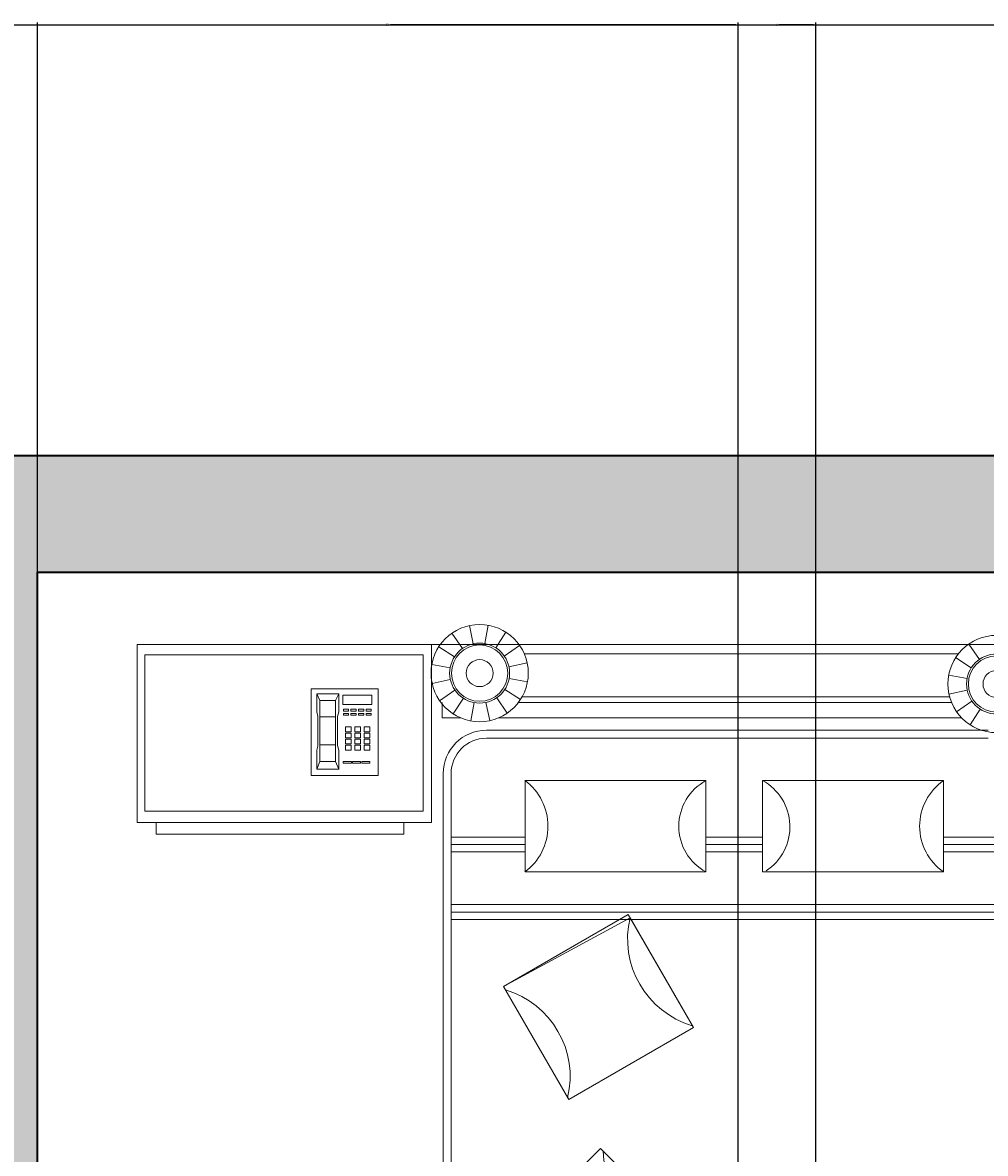
# Model space of a CAD drawing. Units: inches. Extents: x 2070 to 4408, y 1595 to 4269.
# Tile 13 of 20: x 2111 to 2185, y 2238 to 2325. Entities that reach past the tile are written whole.
import ezdxf

# ---------------------------------------------------------------- set-up
doc = ezdxf.new("R2010")
doc.units = ezdxf.units.IN
for name, color, linetype, lineweight in [('A-ANNO-DIMS', 2, 'Continuous', 18), ('A-FURN', 8, 'Continuous', 18), ('A-WALL', 7, 'Continuous', 35)]:
    doc.layers.add(name, color=color, linetype=linetype, lineweight=lineweight)
doc.layers.add('A-WALL-PATT', color=18, linetype='Continuous', lineweight=13, true_color=0x000000)
doc.styles.get("Standard").update_dxf_attribs({"font": 'arial.ttf'})
doc.dimstyles.get("Standard").update_dxf_attribs({"dimtxt": 0.18, "dimasz": 0.18, "dimexe": 0.18, "dimexo": 0.0625, "dimgap": 0.09, "dimtad": 0, "dimtih": 1, "dimtoh": 1, "dimdec": 4, "dimzin": 0, "dimdsep": 46, "dimtxsty": 'Standard', "dimcen": 0.09, "dimadec": 0, "dimazin": 0, "dimtfac": 1, "dimtdec": 4, "dimtofl": 0, "dimtmove": 0, "dimatfit": 3, "dimfxl": 1, "dimtolj": 1, "dimtzin": 0, "dimarcsym": 0})

# ---------------------------------------------------------------- blocks, each defined once
blk = doc.blocks.new('A$C18EB7ED0')
for p, q in [((0.8076, 2.1998), (0.8172, 2.1555)), ((0.8537, 2.2006), (0.8456, 2.1559)), ((0.7653, 2.1814), (0.7911, 2.1442)), ((0.8966, 2.1836), (0.8721, 2.1455)), ((0, 2.1539), (2.8801, 2.1539)), ((0, 1.7209), (0, 2.1539)), ((0.7156, 2.1539), (0.7156, 1.7209)), ((0.7332, 2.1483), (0.7713, 2.1237)), ((0.9298, 2.1515), (0.8925, 2.1257)), ((2.022, 2.155), (2.0478, 2.1177)), ((0.0187, 2.129), (0.695, 2.129)), ((0.0187, 1.7489), (0.0187, 2.129)), ((0.695, 2.129), (0.695, 1.7489)), ((0.941, 2.1314), (1.9968, 2.1314)), ((1.9899, 2.1218), (2.028, 2.0973)), ((0.7162, 2.1054), (0.7608, 2.0973)), ((0.9481, 2.1092), (0.9038, 2.0996)), ((0.717, 2.0593), (0.7613, 2.0688)), ((0.9489, 2.0631), (0.9043, 2.0712)), ((1.973, 2.0789), (2.0176, 2.0708)), ((0.5857, 2.0461), (0.4227, 2.0461)), ((0.4227, 2.0461), (0.4227, 1.8353)), ((0.5857, 1.8353), (0.5857, 2.0461)), ((0.7353, 2.0169), (0.7726, 2.0427)), ((0.9319, 2.0202), (0.8938, 2.0447)), ((1.9737, 2.0328), (2.0181, 2.0424)), ((0.4366, 2.0335), (0.4439, 2.018)), ((0.4903, 2.0335), (0.4366, 2.0335)), ((0.4366, 2.0335), (0.4366, 1.9902)), ((0.4824, 2.018), (0.4439, 2.018)), ((0.4824, 2.018), (0.4439, 2.018)), ((0.4439, 2.018), (0.4439, 1.8697)), ((0.4824, 2.018), (0.4903, 2.0335)), ((0.4824, 1.8697), (0.4824, 2.018)), ((0.4903, 1.9902), (0.4903, 2.0338)), ((0.5706, 2.0307), (0.4996, 2.0307)), ((0.4996, 2.0307), (0.4996, 2.0082)), ((0.4996, 2.0082), (0.5706, 2.0082)), ((0.5706, 2.0082), (0.5706, 2.0307)), ((0.7411, 2.0132), (0.7411, 1.9754)), ((0.7685, 1.9849), (0.7931, 2.023)), ((0.8114, 1.9679), (0.8195, 2.0125)), ((0.8575, 1.9687), (0.848, 2.013)), ((0.8999, 1.987), (0.8741, 2.0243)), ((1.9798, 2.0132), (0.9271, 2.0132)), ((1.9752, 2.0268), (0.9359, 2.0268)), ((1.9921, 1.9905), (2.0294, 2.0163)), ((0.4366, 1.9902), (0.4391, 1.9789)), ((0.4903, 1.9902), (0.4871, 1.9789)), ((0.514, 1.9963), (0.5013, 1.9963)), ((0.5013, 1.9963), (0.5013, 1.992)), ((0.5013, 1.992), (0.514, 1.992)), ((0.514, 1.9864), (0.5013, 1.9864)), ((0.5013, 1.9864), (0.5013, 1.9821)), ((0.5013, 1.9821), (0.514, 1.9821)), ((0.514, 1.992), (0.514, 1.9963)), ((0.514, 1.9821), (0.514, 1.9864)), ((0.5324, 1.9963), (0.5196, 1.9963)), ((0.5196, 1.9963), (0.5196, 1.992)), ((0.5196, 1.992), (0.5324, 1.992)), ((0.5324, 1.9864), (0.5196, 1.9864)), ((0.5196, 1.9864), (0.5196, 1.9821)), ((0.5196, 1.9821), (0.5324, 1.9821)), ((0.5324, 1.992), (0.5324, 1.9963)), ((0.5324, 1.9821), (0.5324, 1.9864)), ((0.5507, 1.9963), (0.538, 1.9963)), ((0.538, 1.9963), (0.538, 1.992)), ((0.538, 1.992), (0.5507, 1.992)), ((0.5507, 1.9864), (0.538, 1.9864)), ((0.538, 1.9864), (0.538, 1.9821)), ((0.538, 1.9821), (0.5507, 1.9821)), ((0.5507, 1.992), (0.5507, 1.9963)), ((0.5507, 1.9821), (0.5507, 1.9864)), ((0.5691, 1.9963), (0.5564, 1.9963)), ((0.5564, 1.9963), (0.5564, 1.992)), ((0.5564, 1.992), (0.5691, 1.992)), ((0.5691, 1.9864), (0.5564, 1.9864)), ((0.5564, 1.9864), (0.5564, 1.9821)), ((0.5564, 1.9821), (0.5691, 1.9821)), ((0.5691, 1.992), (0.5691, 1.9963)), ((0.5691, 1.9821), (0.5691, 1.9864)), ((2.0252, 1.9584), (2.0498, 1.9965)), ((0.4391, 1.9789), (0.4391, 1.9067)), ((0.4824, 1.978), (0.4439, 1.978)), ((0.4871, 1.9789), (0.4871, 1.908)), ((0.52, 1.9534), (0.5062, 1.9534)), ((0.5062, 1.9534), (0.5062, 1.9417)), ((0.52, 1.9417), (0.52, 1.9534)), ((0.5426, 1.9534), (0.5288, 1.9534)), ((0.5288, 1.9534), (0.5288, 1.9417)), ((0.5426, 1.9417), (0.5426, 1.9534)), ((0.5659, 1.9534), (0.5521, 1.9534)), ((0.5521, 1.9534), (0.5521, 1.9417)), ((0.5659, 1.9417), (0.5659, 1.9534)), ((0.7411, 1.9754), (0.7863, 1.9754)), ((0.8788, 1.9754), (2.0045, 1.9754)), ((0.5062, 1.9417), (0.52, 1.9417)), ((0.52, 1.9385), (0.5062, 1.9385)), ((0.5062, 1.9385), (0.5062, 1.9269)), ((0.5062, 1.9269), (0.52, 1.9269)), ((0.52, 1.9269), (0.52, 1.9385)), ((0.5288, 1.9417), (0.5426, 1.9417)), ((0.5426, 1.9385), (0.5288, 1.9385)), ((0.5288, 1.9385), (0.5288, 1.9269)), ((0.5288, 1.9269), (0.5426, 1.9269)), ((0.5426, 1.9269), (0.5426, 1.9385)), ((0.5521, 1.9417), (0.5659, 1.9417)), ((0.5659, 1.9385), (0.5521, 1.9385)), ((0.5521, 1.9385), (0.5521, 1.9269)), ((0.5521, 1.9269), (0.5659, 1.9269)), ((0.5659, 1.9269), (0.5659, 1.9385)), ((2.0691, 1.9452), (0.8491, 1.9452)), ((2.0691, 1.926), (0.8491, 1.926)), ((0.4391, 1.9067), (0.4366, 1.8971)), ((0.4366, 1.8971), (0.4366, 1.8504)), ((0.4439, 1.9101), (0.4824, 1.9101)), ((0.4871, 1.908), (0.4903, 1.8971)), ((0.4903, 1.8499), (0.4903, 1.8971)), ((0.52, 1.9237), (0.5062, 1.9237)), ((0.5062, 1.9237), (0.5062, 1.9121)), ((0.5062, 1.9121), (0.52, 1.9121)), ((0.52, 1.9089), (0.5062, 1.9089)), ((0.5062, 1.9089), (0.5062, 1.8972)), ((0.5062, 1.8972), (0.52, 1.8972)), ((0.52, 1.9121), (0.52, 1.9237)), ((0.52, 1.8972), (0.52, 1.9089)), ((0.5426, 1.9237), (0.5288, 1.9237)), ((0.5288, 1.9237), (0.5288, 1.9121)), ((0.5288, 1.9121), (0.5426, 1.9121)), ((0.5426, 1.9089), (0.5288, 1.9089)), ((0.5288, 1.9089), (0.5288, 1.8972)), ((0.5288, 1.8972), (0.5426, 1.8972)), ((0.5426, 1.9121), (0.5426, 1.9237)), ((0.5426, 1.8972), (0.5426, 1.9089)), ((0.5659, 1.9237), (0.5521, 1.9237)), ((0.5521, 1.9237), (0.5521, 1.9121)), ((0.5521, 1.9121), (0.5659, 1.9121)), ((0.5659, 1.9089), (0.5521, 1.9089)), ((0.5521, 1.9089), (0.5521, 1.8972)), ((0.5521, 1.8972), (0.5659, 1.8972)), ((0.5659, 1.9121), (0.5659, 1.9237)), ((0.5659, 1.8972), (0.5659, 1.9089)), ((0.4439, 1.8697), (0.4366, 1.8504)), ((0.4824, 1.8697), (0.4439, 1.8697)), ((0.4439, 1.8697), (0.4824, 1.8697)), ((0.4903, 1.8504), (0.4824, 1.8697)), ((0.5208, 1.8697), (0.5009, 1.8697)), ((0.5009, 1.8697), (0.5009, 1.8657)), ((0.5208, 1.8657), (0.5208, 1.8697)), ((0.5433, 1.8697), (0.5234, 1.8697)), ((0.5234, 1.8697), (0.5234, 1.8657)), ((0.5433, 1.8657), (0.5433, 1.8697)), ((0.5658, 1.8697), (0.546, 1.8697)), ((0.546, 1.8697), (0.546, 1.8657)), ((0.5658, 1.8657), (0.5658, 1.8697)), ((0.4366, 1.8504), (0.4903, 1.8504)), ((0.5009, 1.8657), (0.5208, 1.8657)), ((0.5234, 1.8657), (0.5433, 1.8657)), ((0.546, 1.8657), (0.5658, 1.8657)), ((0.4227, 1.8353), (0.5857, 1.8353)), ((0.7439, 1.8401), (0.7439, 0.1052)), ((0.7632, 1.8401), (0.7632, 0.1052)), ((0.9429, 1.8231), (1.3829, 1.8231)), ((0.9429, 1.601), (0.9429, 1.8231)), ((1.3829, 1.8231), (1.3829, 1.601)), ((1.5207, 1.601), (1.5207, 1.8231)), ((1.5207, 1.8231), (1.9608, 1.8231)), ((1.9608, 1.8231), (1.9608, 1.601)), ((0.695, 1.7489), (0.0187, 1.7489)), ((0.7156, 1.7209), (0, 1.7209)), ((0, 1.7209), (0.6483, 1.7209)), ((0.0462, 1.6929), (0.0462, 1.7209)), ((0.6483, 1.7209), (0.6483, 1.6929)), ((0.6483, 1.6929), (0.0462, 1.6929)), ((0.7632, 1.6858), (0.9429, 1.6858)), ((1.3829, 1.6858), (1.5207, 1.6858)), ((1.9608, 1.6858), (2.155, 1.6858)), ((0.7632, 1.6678), (0.9429, 1.6678)), ((0.7632, 1.6498), (0.9429, 1.6498)), ((1.3829, 1.6678), (1.5207, 1.6678)), ((1.3829, 1.6498), (1.5207, 1.6498)), ((1.9608, 1.6678), (2.155, 1.6678)), ((1.9608, 1.6498), (2.155, 1.6498)), ((1.3829, 1.601), (0.9429, 1.601)), ((1.9608, 1.601), (1.5207, 1.601)), ((0.7632, 1.5215), (2.155, 1.5215)), ((0.7632, 1.5035), (2.155, 1.5035)), ((0.7632, 1.4855), (2.155, 1.4855)), ((0.8904, 1.3226), (1.1935, 1.4976)), ((0.8904, 1.3226), (1.1982, 1.4894)), ((1.1935, 1.4976), (1.3524, 1.2224)), ((1.1982, 1.4894), (1.3524, 1.2224)), ((1.0493, 1.0474), (0.8904, 1.3226)), ((1.0493, 1.0474), (0.8904, 1.3226)), ((1.3524, 1.2224), (1.0493, 1.0474)), ((1.3524, 1.2224), (1.0493, 1.0474)), ((0.8789, 0.6811), (1.1264, 0.9286)), ((0.8789, 0.6811), (1.1264, 0.9286)), ((1.1264, 0.9286), (1.3473, 0.7077)), ((1.1264, 0.9286), (1.3511, 0.7039))]:
    blk.add_line(p, q)
for centre, radius in [((0.8326, 2.0842), 0.1182), ((2.0893, 2.0578), 0.1182), ((0.8326, 2.0842), 0.0729), ((0.8326, 2.0842), 0.0684), ((0.8326, 2.0842), 0.0328), ((2.0893, 2.0578), 0.0729), ((2.0893, 2.0578), 0.0684), ((2.0893, 2.0578), 0.0328)]:
    blk.add_circle(centre, radius)
for centre, radius, start, end in [((0.8491, 1.8401), 0.1052, 90, 180), ((0.8491, 1.8401), 0.0859, 90, 180), ((0.8604, 1.712), 0.1383, 306.5959, 53.4041), ((1.4431, 1.712), 0.1263, 118.4619, 241.5381), ((1.4584, 1.7106), 0.1286, 303.4023, 61.0264), ((2.0371, 1.712), 0.1347, 124.5027, 235.4973), ((1.4126, 1.4383), 0.2204, 166.5879, 253.4121), ((0.8322, 1.1031), 0.2204, 346.5879, 73.4121), ((1.3534, 0.928), 0.2204, 181.5879, 268.4121)]:
    blk.add_arc(centre, radius, start, end)
blk = doc.blocks.new('*D23')
at = {"layer": 'A-ANNO-DIMS', "color": 0, "lineweight": -2, "transparency": 16777216}
for p, q in [((2103.196, 2291.462), (2103.196, 2324.76)), ((2455.196, 2291.462), (2455.196, 2324.76)), ((2103.376, 2324.579), (2278.908, 2324.579)), ((2455.016, 2324.579), (2279.484, 2324.579))]:
    blk.add_line(p, q, dxfattribs=at)
at = {"layer": 'A-ANNO-DIMS', "color": 0, "transparency": 16777216}
for points in [[(2103.376, 2324.61), (2103.376, 2324.55), (2103.196, 2324.579)], [(2455.016, 2324.61), (2455.016, 2324.55), (2455.196, 2324.579)]]:
    blk.add_solid(points, dxfattribs=at)
at = {"layer": 'Defpoints', "color": 0, "transparency": 16777216}
for p in [(2455.196, 2324.579), (2103.196, 2291.399), (2455.196, 2291.399)]:
    blk.add_point(p, dxfattribs=at)
at = {"layer": 'A-ANNO-DIMS', "color": 0, "transparency": 16777216, "insert": (2279.196, 2324.579), "char_height": 0.18, "attachment_point": 5}
blk.add_mtext('\\A1;352', dxfattribs=at)
blk = doc.blocks.new('*D24')
at = {"layer": 'A-ANNO-DIMS', "color": 0, "lineweight": -2, "transparency": 16777216}
for p, q in [((2103.133, 2291.4), (2069.836, 2291.4)), ((2070.016, 2291.22), (2070.016, 1960.081)), ((2070.016, 1628.58), (2070.016, 1959.718)), ((2336.133, 1628.4), (2069.836, 1628.4))]:
    blk.add_line(p, q, dxfattribs=at)
at = {"layer": 'A-ANNO-DIMS', "color": 0, "transparency": 16777216}
for points in [[(2069.986, 2291.22), (2070.046, 2291.22), (2070.016, 2291.4)], [(2069.986, 1628.58), (2070.046, 1628.58), (2070.016, 1628.4)]]:
    blk.add_solid(points, dxfattribs=at)
at = {"layer": 'Defpoints', "color": 0, "transparency": 16777216}
for p in [(2070.016, 2291.4), (2103.196, 2291.4), (2336.196, 1628.4)]:
    blk.add_point(p, dxfattribs=at)
at = {"layer": 'A-ANNO-DIMS', "color": 0, "transparency": 16777216, "insert": (2070.016, 1959.899), "char_height": 0.18, "attachment_point": 5}
blk.add_mtext('\\A1;663', dxfattribs=at)
blk = doc.blocks.new('*D28')
at = {"layer": 'A-ANNO-DIMS', "color": 0, "lineweight": -2, "transparency": 16777216}
for p, q in [((2166.196, 2000.462), (2166.196, 2324.76)), ((2172.196, 2000.462), (2172.196, 2324.76)), ((2166.376, 2324.579), (2169.047, 2324.579)), ((2172.016, 2324.579), (2169.345, 2324.579))]:
    blk.add_line(p, q, dxfattribs=at)
at = {"layer": 'A-ANNO-DIMS', "color": 0, "transparency": 16777216}
for points in [[(2166.376, 2324.61), (2166.376, 2324.55), (2166.196, 2324.579)], [(2172.016, 2324.61), (2172.016, 2324.55), (2172.196, 2324.579)]]:
    blk.add_solid(points, dxfattribs=at)
at = {"layer": 'Defpoints', "color": 0, "transparency": 16777216}
for p in [(2172.196, 2324.579), (2166.196, 2000.399), (2172.196, 2000.399)]:
    blk.add_point(p, dxfattribs=at)
at = {"layer": 'A-ANNO-DIMS', "color": 0, "transparency": 16777216, "insert": (2169.196, 2324.579), "char_height": 0.18, "attachment_point": 5}
blk.add_mtext('\\A1;6', dxfattribs=at)
blk = doc.blocks.new('*D31')
at = {"layer": 'A-ANNO-DIMS', "color": 0, "lineweight": -2, "transparency": 16777216}
for p, q in [((2112.196, 2000.462), (2112.196, 2324.76)), ((2166.196, 2000.462), (2166.196, 2324.76)), ((2112.376, 2324.579), (2138.977, 2324.579)), ((2166.016, 2324.579), (2139.415, 2324.579))]:
    blk.add_line(p, q, dxfattribs=at)
at = {"layer": 'A-ANNO-DIMS', "color": 0, "transparency": 16777216}
for points in [[(2112.376, 2324.61), (2112.376, 2324.55), (2112.196, 2324.579)], [(2166.016, 2324.61), (2166.016, 2324.55), (2166.196, 2324.579)]]:
    blk.add_solid(points, dxfattribs=at)
at = {"layer": 'Defpoints', "color": 0, "transparency": 16777216}
for p in [(2166.196, 2324.579), (2112.196, 2000.399), (2166.196, 2000.399)]:
    blk.add_point(p, dxfattribs=at)
at = {"layer": 'A-ANNO-DIMS', "color": 0, "transparency": 16777216, "insert": (2139.196, 2324.579), "char_height": 0.18, "attachment_point": 5}
blk.add_mtext('\\A1;54', dxfattribs=at)

msp = doc.modelspace()

# ---------------------------------------------------------------- hatches: boundary and pattern name
at = {"layer": 'A-WALL-PATT'}
h = msp.add_hatch(color=256, dxfattribs=at)
h.dxf.hatch_style = 1
h.paths.add_polyline_path([(2346.196, 2218.3995), (2346.196, 2282.3995), (2340.196, 2282.3995), (2340.196, 2212.3995), (2345.5866, 2212.3995), (2346.196, 2212.3995)], flags=0)
h.paths.add_polyline_path([(2245.196, 2282.3995), (2239.196, 2282.3995), (2239.196, 2186.3995), (2244.5866, 2186.3995), (2245.196, 2186.3995)], flags=0)
h.paths.add_polyline_path([(2340.196, 2230.6455), (2245.196, 2230.6455), (2245.196, 2224.6455), (2340.196, 2224.6455)], flags=0)
h.paths.add_polyline_path([(2245.196, 2150.3995), (2239.196, 2150.3995), (2164.4362, 2150.3995), (2164.4362, 2144.3995), (2239.196, 2144.3995), (2239.196, 2086.3995), (2239.196, 2067.2711), (2244.5866, 2067.2711), (2245.196, 2067.2711), (2245.196, 2144.3995)], flags=0)
h.paths.add_polyline_path([(2346.196, 2176.3995), (2340.196, 2176.3995), (2340.196, 2086.3995), (2346.196, 2086.3995), (2346.196, 2125.318)], flags=0)
h.paths.add_polyline_path([(2446.196, 2086.3995), (2346.196, 2086.3995), (2340.196, 2086.3995), (2340.196, 2080.3995), (2446.196, 2080.3995)], flags=0)
h.paths.add_polyline_path([(2455.196, 2291.3995), (2103.196, 2291.3995), (2103.196, 1699.3995), (2336.196, 1699.3995), (2336.196, 1628.3995), (2345.196, 1628.3995), (2446.196, 1628.3995), (2454.8846, 1628.3995), (2454.8846, 1699.3995)])
h.paths.add_polyline_path([(2446.196, 2282.3995), (2446.196, 2218.3995), (2446.196, 2212.3995), (2446.196, 2086.3995), (2446.196, 2080.3995), (2446.196, 1708.3995), (2446.196, 1637.3995), (2345.196, 1637.3995), (2345.196, 1699.3995), (2345.196, 1708.3995), (2336.196, 1708.3995), (2112.196, 1708.3995), (2112.196, 2282.3995), (2239.196, 2282.3995), (2245.196, 2282.3995), (2356.196, 2282.3995)], flags=16)
h.paths.add_polyline_path([(2245.196, 2150.3995), (2245.196, 2144.3995), (2245.196, 2067.2711), (2244.5866, 2067.2711), (2239.196, 2067.2711), (2239.196, 2065.6988), (2203.2929, 2065.6988, 0.4014527), (2239.196, 2031.3337), (2244.5866, 2031.3337), (2245.196, 2031.2711), (2245.196, 1924.1525), (2239.196, 1924.1525), (2239.196, 1922.5803), (2203.2929, 1922.5803, 0.4014527), (2239.196, 1888.2151), (2244.5866, 1888.2151), (2245.196, 1888.1525), (2245.196, 1748.3995), (2339.196, 1748.4621, -0.4014527), (2303.2929, 1782.8272), (2303.2585, 1782.8272), (2303.2585, 1784.3995), (2339.196, 1784.3995), (2339.196, 1877.2067), (2291.196, 1877.2067), (2291.196, 1883.2067), (2291.196, 1946.3995), (2291.196, 1952.3995), (2291.196, 2086.3995), (2297.196, 2086.3995), (2302.196, 2086.3995), (2302.196, 2081.0259), (2303.7633, 2081.0259), (2303.7633, 2080.3995), (2338.0148, 2080.3995, 0.0043713), (2338.0203, 2081.0259), (2338.0203, 2086.3995), (2340.196, 2086.3995), (2340.196, 2176.4621), (2345.5866, 2176.4621, 0.4014527), (2381.4896, 2210.8272), (2345.5866, 2210.8272), (2345.5866, 2212.3995), (2340.196, 2212.3995), (2340.196, 2224.6455), (2245.196, 2224.6455), (2245.196, 2186.3995), (2244.5866, 2186.3995), (2239.196, 2186.3995), (2239.196, 2184.8272), (2203.2929, 2184.8272, 0.4014527), (2239.196, 2150.4621), (2244.5866, 2150.4621)], flags=0)
h.paths.add_polyline_path([(2346.196, 2282.3995), (2346.196, 2218.3995), (2377.1813, 2218.3995), (2377.1813, 2212.3995), (2346.196, 2212.3995), (2345.5866, 2212.3995), (2340.196, 2212.3995), (2340.196, 2224.6455), (2245.196, 2224.6455), (2245.196, 2230.6455), (2245.196, 2282.3995), (2292.696, 2256.5225), (2340.196, 2282.3995)], flags=0)
h.paths.add_polyline_path([(2346.196, 2086.3995), (2340.196, 2086.3995), (2340.196, 2080.3995), (2446.196, 2080.3995), (2431.196, 2016.3995), (2446.196, 1952.3995), (2412.196, 1952.3995), (2412.196, 2080.3995), (2340.196, 2080.3995), (2340.196, 2086.3995), (2340.196, 2176.3995), (2346.196, 2176.3995), (2346.196, 2125.318)], flags=0)
h.paths.add_polyline_path([(2186.508, 2270.0471, -0.0375529), (2186.9712, 2269.8581), (2186.9164, 2270.112, -0.0275912)], flags=0)
h.paths.add_polyline_path([(2183.955, 2273.7766, 1), (2188.2945, 2273.7766, 1)], flags=0)
h.paths.add_polyline_path([(2142.5261, 2274.6158, -0.0370754), (2142.5672, 2275.1696), (2142.5672, 2276.826), (2119.8759, 2276.826), (2119.8759, 2263.0962), (2140.4332, 2263.0962), (2142.5672, 2263.0962), (2142.5672, 2274.0621, -0.0370754)], flags=0)
h.paths.add_polyline_path([(2209.8974, 2263.0962), (2209.8974, 2262.2079), (2190.8042, 2262.2079), (2190.8042, 2263.0962)], flags=0)
h.paths.add_polyline_path([(2210.6382, 2276.1833), (2210.6382, 2263.9844), (2190.2185, 2263.9844), (2190.2185, 2276.1833)], flags=0)
h.paths.add_polyline_path([(2188.4362, 2273.7766, -1), (2183.8133, 2273.7766, -1)], flags=0)
h.paths.add_polyline_path([(2245.196, 2150.3995), (2245.196, 2144.3995), (2245.196, 2067.2711), (2239.196, 2067.2711), (2239.196, 2080.3995), (2172.196, 2080.3995), (2172.196, 2000.3995), (2239.196, 2000.3995), (2239.196, 1940.3995), (2159.0187, 1940.3995), (2123.0187, 1940.3995), (2112.196, 1940.3995), (2112.196, 1946.3995), (2123.0187, 1946.3995), (2123.0187, 1982.2238), (2124.586, 1982.2238), (2124.586, 1982.1895, -0.4014527), (2158.8429, 1946.3995), (2159.0187, 1946.3995), (2239.196, 1946.3995), (2239.196, 1994.3995), (2112.196, 1994.3995), (2112.196, 2000.3995), (2139.196, 2040.3995), (2112.196, 2080.3995), (2112.196, 2086.3995), (2239.196, 2086.3995), (2239.196, 2144.3995), (2209.5809, 2144.3995), (2209.5809, 2136.3995), (2203.0809, 2136.3995), (2205.0809, 2130.3996, -0.7025712), (2199.081, 2116.3995, -0.7025621), (2193.0809, 2130.3994), (2195.0809, 2136.3995), (2192.0809, 2136.3995), (2192.0809, 2134.8995), (2189.0809, 2134.8995), (2189.0809, 2135.8995), (2191.0809, 2135.8995), (2191.0809, 2136.3995), (2188.5809, 2136.3995), (2188.5809, 2144.3995), (2164.2481, 2144.3995, -0.3938585), (2130.0035, 2109.5491), (2130.0035, 2109.5147), (2128.4362, 2109.5147), (2128.4362, 2144.3995), (2112.196, 2144.3995), (2112.196, 2150.3995), (2128.4362, 2150.3995), (2128.4362, 2150.7127), (2164.4362, 2150.7127), (2164.4362, 2150.3995), (2239.196, 2150.3995)], flags=0)
h.paths.add_polyline_path([(2188.2075, 2266.8735), (2188.2075, 2211.8632, -0.4142136), (2185.4833, 2209.1391), (2146.7995, 2209.1391, -0.4142136), (2144.0754, 2211.8632), (2144.0754, 2266.8735, -0.4142136), (2146.7995, 2269.5976), (2185.4833, 2269.5976, -0.4142136)], flags=0)
h.paths.add_polyline_path([(2185.0844, 2273.7766, -1), (2187.1651, 2273.7766, -1)], flags=0)
h.paths.add_polyline_path([(2182.0486, 2259.2932), (2168.0953, 2259.2932), (2168.0953, 2260.8424), (2163.7261, 2260.8424), (2163.7261, 2259.2932), (2149.7727, 2259.2932), (2149.7727, 2266.3352), (2163.7261, 2266.3352), (2163.7261, 2261.9839), (2168.0953, 2261.9839), (2168.0953, 2266.3352), (2182.0486, 2266.3352)], flags=0)
h.paths.add_polyline_path([(2148.2585, 2250.2051), (2153.0615, 2241.8861, 0.3980705)], flags=0)
h.paths.add_polyline_path([(2162.7572, 2247.2885), (2153.1461, 2241.7396), (2148.1083, 2250.4653), (2157.7194, 2256.0142)], flags=0)
h.paths.add_polyline_path([(2162.6726, 2247.4351, -0.392862), (2157.8415, 2255.6313), (2157.6431, 2255.6313), (2157.8696, 2255.7541)], flags=0)
h.paths.add_polyline_path([(2164.2604, 2145.339), (2164.4362, 2144.3995), (2164.4362, 2150.3995), (2164.2604, 2150.7127)], flags=0)
h.paths.add_polyline_path([(2208.5809, 2142.6495), (2208.5809, 2138.3995, -0.4142136), (2207.8309, 2137.3995), (2190.5809, 2137.3995, -0.4142136), (2189.5809, 2138.1495), (2189.5809, 2142.3995, -0.4142136), (2190.3309, 2143.3995), (2207.5809, 2143.3995, -0.4142136)], flags=0)
h.paths.add_polyline_path([(2147.957, 2229.9119), (2154.7494, 2223.1195, 0.3980705)], flags=0)
h.paths.add_polyline_path([(2162.7165, 2230.8473), (2154.8691, 2222.9998), (2147.7446, 2230.1244), (2155.592, 2237.9718)], flags=0)
h.paths.add_polyline_path([(2162.5969, 2230.9669, -0.3980705), (2155.8044, 2237.7594)], flags=0)
h.paths.add_polyline_path([(2391.8776, 2049.9192), (2408.5766, 2049.9192), (2408.5766, 2033.2202), (2408.5766, 1983.123), (2408.5766, 1966.4239), (2391.8776, 1966.4239), (2391.8776, 1983.123), (2341.7804, 1983.123), (2341.7804, 2033.2202), (2391.8776, 2033.2202)], flags=0)
h.paths.add_polyline_path([(2144.1055, 2274.6158, 1), (2148.445, 2274.6158, 1)], flags=0)
h.paths.add_polyline_path([(2148.5867, 2274.6158, -1), (2143.9638, 2274.6158, -1)], flags=0)
h.paths.add_polyline_path([(2145.2349, 2274.6158, -1), (2147.3156, 2274.6158, -1)], flags=0)
edge = h.paths.add_edge_path(flags=0)
edge.add_ellipse((2400.5951, 2040.9436), major_axis=(-4.5109, 0), ratio=0.9754478, start_angle=180, end_angle=270, ccw=False)
edge.add_ellipse((2400.5951, 2040.9436), major_axis=(-4.5109, 0), ratio=0.9754478, start_angle=90, end_angle=180, ccw=False)
edge.add_ellipse((2400.5951, 2040.9436), major_axis=(-4.5109, 0), ratio=0.9754478, start_angle=0, end_angle=90, ccw=False)
edge.add_ellipse((2400.5951, 2040.9436), major_axis=(-4.5109, 0), ratio=0.9754478, start_angle=270, end_angle=360, ccw=False)
h.paths.add_polyline_path([(2199.0809, 2117.3995, -0.7345297), (2195.0809, 2130.3995), (2203.081, 2130.3995, -0.7345333)], flags=0)
h.paths.add_polyline_path([(2141.9147, 2276.0353), (2141.9147, 2263.9844), (2120.4685, 2263.9844), (2120.4685, 2276.0353)], flags=0)
h.paths.add_polyline_path([(2138.4481, 2273.4072), (2138.4481, 2266.7226), (2133.2801, 2266.7226), (2133.2801, 2273.4072)], flags=0)
h.paths.add_polyline_path([(2137.9691, 2272.9175), (2137.9691, 2272.204), (2135.4229, 2272.204), (2135.4229, 2271.6329), (2135.3221, 2270.1051), (2135.3221, 2269.0265), (2135.4229, 2268.6811), (2135.4229, 2267.2011), (2133.7212, 2267.2011), (2133.7212, 2268.6811), (2133.7983, 2269.9587), (2133.7983, 2271.2758), (2133.7212, 2271.6329), (2133.7212, 2273.0065), (2135.717, 2273.0065), (2135.717, 2272.9175)], flags=0)
h.paths.add_polyline_path([(2137.9215, 2271.8264), (2137.9215, 2271.3786), (2137.5182, 2271.3786), (2136.9355, 2271.3786), (2136.3529, 2271.3786), (2135.7703, 2271.3786), (2135.7703, 2271.8264), (2136.1736, 2271.8264), (2136.7562, 2271.8264), (2137.3389, 2271.8264)], flags=0)
h.paths.add_polyline_path([(2137.9215, 2271.692), (2137.5182, 2271.692), (2136.9355, 2271.513), (2137.3389, 2271.513)], flags=0)
h.paths.add_polyline_path([(2136.3529, 2271.692), (2135.7703, 2271.513), (2136.1736, 2271.513), (2136.7562, 2271.692)], flags=0)
h.paths.add_polyline_path([(2137.9215, 2271.513), (2137.5182, 2271.513), (2136.7562, 2271.747), (2136.7562, 2271.692), (2137.3389, 2271.692)], flags=0)
h.paths.add_polyline_path([(2137.8207, 2270.4664), (2137.8207, 2270.0971), (2137.8207, 2269.627), (2137.8207, 2269.1569), (2137.8207, 2268.6868), (2137.3837, 2268.6868), (2136.6442, 2268.6868), (2135.9271, 2268.6868), (2135.9271, 2269.0562), (2135.9271, 2269.5263), (2135.9271, 2269.9963), (2135.9271, 2270.4664), (2136.3641, 2270.4664), (2137.0812, 2270.4664)], flags=0)
h.paths.add_polyline_path([(2137.3837, 2269.627), (2137.8207, 2269.627), (2137.8207, 2269.5263), (2137.3837, 2269.5263), (2137.3837, 2269.1569), (2137.8207, 2269.1569), (2137.3837, 2269.0562), (2137.3837, 2268.6868), (2137.0812, 2268.6868), (2137.0812, 2269.0562), (2136.6442, 2269.0562), (2136.6442, 2268.6868), (2136.3641, 2268.6868), (2136.3641, 2269.0562), (2135.9271, 2269.0562), (2135.9271, 2269.1569), (2136.3641, 2269.1569), (2136.3641, 2269.5263), (2135.9271, 2269.5263), (2135.9271, 2269.627), (2136.3641, 2269.627), (2136.3641, 2269.9963), (2135.9271, 2269.9963), (2136.3641, 2270.0971), (2136.3641, 2270.4664), (2136.6442, 2270.4664), (2136.6442, 2270.0971), (2137.0812, 2270.0971), (2137.0812, 2270.4664), (2137.3837, 2270.4664), (2137.3837, 2270.0971), (2137.8207, 2270.0971), (2137.3837, 2269.9963)], flags=0)
h.paths.add_polyline_path([(2137.5182, 2271.8264), (2137.5182, 2271.692), (2137.3389, 2271.3786), (2137.3389, 2271.513)], flags=0)
h.paths.add_polyline_path([(2137.8179, 2267.8138), (2137.8179, 2267.6879), (2137.1876, 2267.6879), (2136.4733, 2267.6879), (2135.759, 2267.6879), (2135.759, 2267.8138), (2136.3893, 2267.8138), (2137.1036, 2267.8138)], flags=0)
h.paths.add_polyline_path([(2137.0812, 2269.9963), (2137.0812, 2269.627), (2137.0812, 2269.1569), (2136.6442, 2269.1569), (2136.6442, 2269.5263), (2136.6442, 2269.9963)], flags=0)
h.paths.add_polyline_path([(2136.3529, 2271.8264), (2136.3529, 2271.692), (2136.1736, 2271.3786), (2136.1736, 2271.513)], flags=0)
h.paths.add_polyline_path([(2136.4733, 2267.8138), (2136.4733, 2267.6879), (2136.3893, 2267.6879), (2136.3893, 2267.8138)], flags=0)
h.paths.add_polyline_path([(2407.9087, 2032.5522), (2407.9087, 1983.7909), (2359.81, 1983.7909, -0.0091279), (2359.0575, 1983.7909), (2342.4483, 1983.7909), (2342.4483, 2032.5522)], flags=0)
h.paths.add_polyline_path([(2389.1838, 2023.1358), (2353.7856, 2023.1358), (2353.7856, 1985.4867, -0.0921038), (2350.2788, 1988.655), (2350.2788, 2026.6426), (2389.1838, 2026.6426)], flags=0)
h.paths.add_polyline_path([(2352.6166, 2024.3048), (2351.4477, 2024.3048), (2351.4477, 2025.4737), (2352.6166, 2025.4737)], flags=0)
h.paths.add_polyline_path([(2399.6319, 2026.7589), (2404.3661, 2026.7589, -0.4142136), (2407.0379, 2024.087), (2407.0379, 2013.4908, -0.4142136), (2404.3661, 2010.819), (2399.6319, 2010.819, -0.4142136), (2396.96, 2013.4908), (2396.96, 2024.087, -0.4142136)], flags=0)
h.paths.add_polyline_path([(2399.6319, 2026.0909), (2404.3661, 2026.0909, -0.4142136), (2406.37, 2024.087), (2406.37, 2013.4908, -0.4142136), (2404.3661, 2011.487), (2399.6319, 2011.487, -0.4142136), (2397.628, 2013.4908), (2397.628, 2024.087, -0.4142136)], flags=0)
h.paths.add_polyline_path([(2399.6319, 2002.3217), (2404.3661, 2002.3217, -0.4142136), (2407.0379, 1999.6498), (2407.0379, 1989.0536, -0.4142136), (2404.3661, 1986.3818), (2399.6319, 1986.3818, -0.4142136), (2396.96, 1989.0536), (2396.96, 1999.6498, -0.4142136)], flags=0)
h.paths.add_polyline_path([(2399.6319, 2001.6537), (2404.3661, 2001.6537, -0.4142136), (2406.37, 1999.6498), (2406.37, 1989.0536, -0.4142136), (2404.3661, 1987.0497), (2399.6319, 1987.0497, -0.4142136), (2397.628, 1989.0536), (2397.628, 1999.6498, -0.4142136)], flags=0)
edge = h.paths.add_edge_path(flags=0)
edge.add_ellipse((2400.5951, 1975.3996), major_axis=(-4.5109, 0), ratio=0.9754478, start_angle=-180, end_angle=-90, ccw=False)
edge.add_ellipse((2400.5951, 1975.3996), major_axis=(-4.5109, 0), ratio=0.9754478, start_angle=90, end_angle=180, ccw=False)
edge.add_ellipse((2400.5951, 1975.3996), major_axis=(-4.5109, 0), ratio=0.9754478, start_angle=0, end_angle=90, ccw=False)
edge.add_ellipse((2400.5951, 1975.3996), major_axis=(-4.5109, 0), ratio=0.9754478, start_angle=-90, end_angle=0, ccw=False)
h.paths.add_polyline_path([(2345.196, 1910.3995), (2366.4386, 1910.3995), (2366.4386, 1925.4555), (2392.3856, 1925.4555), (2392.3856, 1933.5025), (2400.1399, 1925.4555), (2392.3856, 1919.8795), (2392.3856, 1925.4555), (2366.4386, 1925.4555), (2366.4386, 1910.3995), (2381.196, 1910.3995), (2405.196, 1910.3995), (2405.196, 1898.3995), (2446.196, 1898.3995), (2446.196, 1886.3995), (2405.196, 1886.3995), (2405.196, 1874.3995), (2446.196, 1874.3995), (2446.196, 1862.3995), (2405.196, 1862.3995), (2405.196, 1850.3995), (2446.196, 1850.3995), (2446.196, 1838.3995), (2405.196, 1838.3995), (2405.196, 1826.3995), (2446.196, 1826.3995), (2446.196, 1814.3995), (2405.196, 1814.3995), (2405.196, 1802.3995), (2446.196, 1802.3995), (2446.196, 1798.3995), (2446.196, 1792.3995), (2405.196, 1792.3995), (2405.196, 1910.3995), (2381.196, 1910.3995), (2381.196, 1792.3995), (2345.196, 1792.3995)], flags=0)
h.paths.add_polyline_path([(2333.0944, 1863.3993, -0.4142136), (2334.7225, 1861.7712), (2334.7225, 1859.329), (2335.2653, 1859.329, -0.4142136), (2337.4361, 1857.1582), (2337.4361, 1843.862, -0.4142136), (2335.2653, 1841.6911, -0.4142136), (2337.4361, 1839.5203), (2337.4361, 1827.5808, -0.4142136), (2335.2653, 1825.41, -0.4142136), (2337.4361, 1823.2392), (2337.4361, 1808.5862, -0.4142136), (2335.2653, 1806.4153), (2334.7225, 1806.4153), (2334.7225, 1803.9732, -0.4142136), (2333.0944, 1802.3451), (2317.356, 1802.3451), (2317.0846, 1802.3451, -0.4142136), (2315.7279, 1803.7018), (2315.7279, 1803.8646), (2313.8284, 1803.8646, -0.4142136), (2311.6576, 1806.0354), (2311.6576, 1823.2015, -0.395976), (2313.6834, 1825.3765, -0.433848), (2311.6576, 1827.2718), (2311.6576, 1839.761, -0.4142136), (2313.5571, 1841.6604), (2313.8284, 1841.6604), (2333.8159, 1841.6604, -0.0421362), (2334.1798, 1841.6911, -0.4142136), (2332.009, 1843.862), (2332.009, 1857.1582, -0.4142136), (2334.1798, 1859.329), (2317.356, 1859.329), (2317.0846, 1859.329, -0.4142136), (2315.7279, 1860.6858), (2315.7279, 1862.0426, -0.4142136), (2317.0846, 1863.3993), (2317.356, 1863.3993)], flags=0)
h.paths.add_polyline_path([(2208.8475, 1848.9818), (2208.8475, 1840.9741, -0.4142136), (2207.0458, 1839.1724), (2206.5453, 1839.1721), (2206.5453, 1838.7218, -0.4098586), (2204.7704, 1836.9203), (2183.7501, 1836.9203, -0.418582), (2181.9216, 1838.7218), (2181.9216, 1839.1721), (2181.421, 1839.1724, -0.4142136), (2179.6193, 1840.9741), (2179.6193, 1848.6817, -0.4406442), (2185.1126, 1854.9874), (2203.3852, 1854.9874, -0.4570796)], flags=0)
h.paths.add_polyline_path([(2204.243, 1848.4815), (2204.243, 1848.4815, 0.4172533), (2202.2204, 1850.4833), (2186.2049, 1850.4833, 0.4111805), (2184.2237, 1848.4815), (2184.2237, 1848.4815, -0.4111807), (2186.2049, 1850.4833), (2202.2204, 1850.4833, -0.4172531)], flags=0)
h.paths.add_polyline_path([(2234.7177, 1830.228), (2234.7176, 1781.6047, -0.4142136), (2233.4381, 1780.3252), (2218.6064, 1780.3252, -0.4142136), (2217.8387, 1781.0929), (2217.8387, 1783.3961, -0.4142136), (2218.6064, 1784.1639), (2218.6065, 1796.9595, -0.4142136), (2219.886, 1798.239, -0.4142136), (2218.6065, 1799.5186), (2218.6065, 1812.3142, -0.4142136), (2219.8861, 1813.5938, -0.4142136), (2218.6065, 1814.8733), (2218.6065, 1827.6689, -0.4142136), (2217.8388, 1828.4367), (2217.8388, 1830.7399, -0.4142136), (2218.6065, 1831.5076), (2233.4382, 1831.5076, -0.4142136)], flags=0)
h.paths.add_polyline_path([(2230.6344, 1827.6689, -0.4142136), (2231.4021, 1826.9012), (2231.4021, 1784.9316, -0.4142136), (2230.6343, 1784.1639), (2221.1853, 1784.1639), (2221.1853, 1827.6689)], flags=0)
h.paths.add_polyline_path([(2222.7208, 1798.239), (2221.6971, 1798.239), (2221.6971, 1813.5938), (2222.7208, 1813.5938)], flags=0)
h.paths.add_polyline_path([(2206.5453, 1773.935), (2206.5453, 1773.4848), (2206.9457, 1773.4848), (2207.0458, 1773.4845, -0.4142136), (2208.8475, 1771.6827), (2208.8475, 1763.675, -0.4422243), (2203.6505, 1757.6695), (2185.3851, 1757.6695, -0.455084), (2179.6193, 1763.9752), (2179.6193, 1771.6827, -0.4142136), (2181.421, 1773.4845), (2181.421, 1773.4848), (2181.9216, 1773.4848), (2181.9216, 1773.935, -0.4098586), (2183.6965, 1775.7366), (2204.7167, 1775.7366, -0.418582)], flags=0)
h.paths.add_polyline_path([(2202.2619, 1762.1736), (2186.2464, 1762.1736, -0.4172531), (2184.2237, 1764.1754), (2184.2237, 1764.1754, 0.4172533), (2186.2464, 1762.1736), (2202.2619, 1762.1736, 0.4111805), (2204.243, 1764.1754), (2204.243, 1764.1754, -0.4111807)], flags=0)
h.paths.add_polyline_path([(2313.0034, 1713.1906), (2312.997, 1713.1697), (2313.0123, 1713.1612)], flags=0)
h.paths.add_polyline_path([(2305.7314, 1721.0488), (2305.6257, 1721.1994), (2305.4853, 1721.084)], flags=0)
h.paths.add_polyline_path([(2307.5562, 1726.1427), (2307.6186, 1726.1026), (2307.5737, 1726.0477), (2308.5692, 1720.6434), (2310.5345, 1721.2985), (2310.5721, 1721.411), (2310.6958, 1721.3523), (2313.8453, 1722.4021), (2314.9351, 1723.8033), (2314.9294, 1723.9165), (2315.0028, 1723.8903), (2313.874, 1722.4389), (2313.8697, 1722.4102), (2308.5692, 1720.6434), (2308.9864, 1720.122), (2309.0665, 1720.0971), (2309.053, 1720.0387), (2310.9235, 1717.7005), (2311.4182, 1717.6259), (2311.2918, 1717.2402), (2312.0655, 1716.2731), (2312.1081, 1716.2606), (2312.0969, 1716.2339), (2308.5692, 1720.6434), (2305.2249, 1717.745), (2305.232, 1717.704), (2305.1665, 1717.6944), (2308.5692, 1720.6434)], flags=0)
h.paths.add_polyline_path([(2288.2072, 1714.3431), (2288.2008, 1714.3222), (2288.216, 1714.3137)], flags=0)
h.paths.add_polyline_path([(2280.9352, 1722.2013), (2280.8295, 1722.3519), (2280.689, 1722.2365)], flags=0)
h.paths.add_polyline_path([(2282.76, 1727.2952), (2282.8224, 1727.2551), (2282.7775, 1727.2002), (2283.773, 1721.7959), (2285.7383, 1722.451), (2285.7759, 1722.5635), (2285.8995, 1722.5048), (2289.0491, 1723.5546), (2290.1389, 1724.9558), (2290.1332, 1725.069), (2290.2065, 1725.0428), (2289.0777, 1723.5915), (2289.0735, 1723.5628), (2283.773, 1721.7959), (2284.1901, 1721.2745), (2284.2703, 1721.2496), (2284.2567, 1721.1913), (2286.1273, 1718.8531), (2286.622, 1718.7785), (2286.4956, 1718.3927), (2287.2692, 1717.4256), (2287.3119, 1717.4131), (2287.3006, 1717.3864), (2283.773, 1721.7959), (2280.4286, 1718.8975), (2280.4357, 1718.8565), (2280.3703, 1718.8469), (2283.773, 1721.7959)], flags=0)
h.paths.add_polyline_path([(2302.0672, 1721.8694), (2301.8205, 1721.8572), (2301.7578, 1722.1787), (2299.415, 1724.5215), (2299.103, 1724.4694), (2299.0662, 1724.8703)], flags=0)
h.paths.add_polyline_path([(2264.5643, 1715.4956), (2264.5579, 1715.4747), (2264.5731, 1715.4662)], flags=0)
h.paths.add_polyline_path([(2257.2923, 1723.3538), (2257.1865, 1723.5044), (2257.0461, 1723.389)], flags=0)
h.paths.add_polyline_path([(2259.117, 1728.4477), (2259.1795, 1728.4077), (2259.1345, 1728.3527), (2260.13, 1722.9484), (2262.0954, 1723.6036), (2262.133, 1723.716), (2262.2566, 1723.6573), (2265.4061, 1724.7071), (2266.4959, 1726.1083), (2266.4902, 1726.2215), (2266.5636, 1726.1953), (2265.4348, 1724.744), (2265.4305, 1724.7153), (2260.13, 1722.9484), (2260.5472, 1722.427), (2260.6273, 1722.4022), (2260.6138, 1722.3438), (2262.4843, 1720.0056), (2262.979, 1719.931), (2262.8526, 1719.5452), (2263.6263, 1718.5781), (2263.6689, 1718.5656), (2263.6577, 1718.5389), (2260.13, 1722.9484), (2256.7857, 1720.05), (2256.7928, 1720.009), (2256.7273, 1719.9994), (2260.13, 1722.9484)], flags=0)
h.paths.add_polyline_path([(2277.2709, 1723.0219), (2277.0243, 1723.0097), (2276.9616, 1723.3312), (2274.6187, 1725.6741), (2274.3067, 1725.6219), (2274.27, 1726.0228)], flags=0)
h.paths.add_polyline_path([(2253.628, 1724.1744), (2253.3814, 1724.1622), (2253.3186, 1724.4838), (2250.9758, 1726.8266), (2250.6638, 1726.7744), (2250.627, 1727.1753)], flags=0)
h.paths.add_polyline_path([(2161.9194, 1715.4956), (2161.913, 1715.4747), (2161.9282, 1715.4662)], flags=0)
h.paths.add_polyline_path([(2154.6474, 1723.3538), (2154.5416, 1723.5044), (2154.4012, 1723.389)], flags=0)
h.paths.add_polyline_path([(2162.7899, 1724.744), (2162.7856, 1724.7153), (2157.4851, 1722.9484), (2157.9023, 1722.427), (2157.9824, 1722.4022), (2157.9689, 1722.3438), (2159.8394, 1720.0056), (2160.3341, 1719.931), (2160.2078, 1719.5452), (2160.9814, 1718.5781), (2161.024, 1718.5656), (2161.0128, 1718.5389), (2157.4851, 1722.9484), (2154.1408, 1720.05), (2154.1479, 1720.009), (2154.0824, 1719.9994), (2157.4851, 1722.9484), (2156.4721, 1728.4477), (2156.5346, 1728.4077), (2156.4896, 1728.3527), (2157.4851, 1722.9484), (2159.4505, 1723.6036), (2159.4881, 1723.716), (2159.6117, 1723.6573), (2162.7612, 1724.7071), (2163.851, 1726.1083), (2163.8453, 1726.2215), (2163.9187, 1726.1953)], flags=0)
h.paths.add_polyline_path([(2150.9831, 1724.1744), (2150.7365, 1724.1622), (2150.6738, 1724.4838), (2148.3309, 1726.8266), (2148.0189, 1726.7744), (2147.9822, 1727.1753)], flags=0)
h.paths.add_polyline_path([(2132.5099, 1716.6482), (2132.5035, 1716.6272), (2132.5187, 1716.6187)], flags=0)
h.paths.add_polyline_path([(2125.2379, 1724.5064), (2125.1322, 1724.6569), (2124.9917, 1724.5415)], flags=0)
h.paths.add_polyline_path([(2133.3804, 1725.8965), (2133.3762, 1725.8678), (2128.0757, 1724.101), (2128.4928, 1723.5795), (2128.5729, 1723.5547), (2128.5594, 1723.4963), (2130.43, 1721.1581), (2130.9246, 1721.0835), (2130.7983, 1720.6977), (2131.5719, 1719.7306), (2131.6146, 1719.7181), (2131.6033, 1719.6914), (2128.0757, 1724.101), (2124.7313, 1721.2025), (2124.7384, 1721.1615), (2124.6729, 1721.1519), (2128.0757, 1724.101), (2127.0626, 1729.6002), (2127.1251, 1729.5602), (2127.0801, 1729.5052), (2128.0757, 1724.101), (2130.041, 1724.7561), (2130.0786, 1724.8685), (2130.2022, 1724.8098), (2133.3517, 1725.8597), (2134.4415, 1727.2608), (2134.4358, 1727.3741), (2134.5092, 1727.3478)], flags=0)
h.paths.add_polyline_path([(2121.5736, 1725.3269), (2121.327, 1725.3148), (2121.2643, 1725.6363), (2118.9214, 1727.9791), (2118.6094, 1727.9269), (2118.5727, 1728.3279)], flags=0)
h.paths.add_polyline_path([(2433.3904, 1646.406), (2433.384, 1646.3851), (2433.3992, 1646.3766)], flags=0)
h.paths.add_polyline_path([(2426.1184, 1654.2642), (2426.0127, 1654.4148), (2425.8722, 1654.2994)], flags=0)
h.paths.add_polyline_path([(2427.9432, 1659.3581), (2428.0056, 1659.318), (2427.9606, 1659.2631), (2428.9562, 1653.8588), (2430.9215, 1654.514), (2430.9591, 1654.6264), (2431.0827, 1654.5677), (2434.2323, 1655.6175), (2435.322, 1657.0187), (2435.3163, 1657.1319), (2435.3897, 1657.1057), (2434.2609, 1655.6544), (2434.2567, 1655.6257), (2428.9562, 1653.8588), (2429.3733, 1653.3374), (2429.4534, 1653.3126), (2429.4399, 1653.2542), (2431.3105, 1650.916), (2431.8051, 1650.8414), (2431.6788, 1650.4556), (2432.4524, 1649.4885), (2432.4951, 1649.476), (2432.4838, 1649.4493), (2428.9562, 1653.8588), (2425.6118, 1650.9604), (2425.6189, 1650.9194), (2425.5535, 1650.9098), (2428.9562, 1653.8588)], flags=0)
h.paths.add_polyline_path([(2376.63, 1645.4912), (2376.6236, 1645.4703), (2376.6388, 1645.4617)], flags=0)
h.paths.add_polyline_path([(2369.358, 1653.3494), (2369.2523, 1653.5), (2369.1118, 1653.3845)], flags=0)
h.paths.add_polyline_path([(2371.1828, 1658.4432), (2371.2452, 1658.4032), (2371.2003, 1658.3482), (2372.1958, 1652.944), (2374.1611, 1653.5991), (2374.1987, 1653.7116), (2374.3224, 1653.6528), (2377.4719, 1654.7027), (2378.5617, 1656.1038), (2378.556, 1656.2171), (2378.6293, 1656.1908), (2377.5005, 1654.7395), (2377.4963, 1654.7108), (2372.1958, 1652.944), (2372.6129, 1652.4225), (2372.6931, 1652.3977), (2372.6795, 1652.3393), (2374.5501, 1650.0011), (2375.0448, 1649.9265), (2374.9184, 1649.5407), (2375.692, 1648.5737), (2375.7347, 1648.5611), (2375.7234, 1648.5344), (2372.1958, 1652.944), (2368.8514, 1650.0456), (2368.8586, 1650.0046), (2368.7931, 1649.995), (2372.1958, 1652.944)], flags=0)
h.paths.add_polyline_path([(2404.0947, 1645.0338), (2404.0883, 1645.0128), (2404.1035, 1645.0043)], flags=0)
h.paths.add_polyline_path([(2396.8227, 1652.892), (2396.717, 1653.0425), (2396.5765, 1652.9271)], flags=0)
h.paths.add_polyline_path([(2398.6475, 1657.9858), (2398.7099, 1657.9458), (2398.665, 1657.8908), (2399.6605, 1652.4866), (2401.6258, 1653.1417), (2401.6634, 1653.2541), (2401.7871, 1653.1954), (2404.9366, 1654.2453), (2406.0264, 1655.6464), (2406.0207, 1655.7596), (2406.094, 1655.7334), (2404.9652, 1654.2821), (2404.961, 1654.2534), (2399.6605, 1652.4866), (2400.0776, 1651.9651), (2400.1578, 1651.9403), (2400.1442, 1651.8819), (2402.0148, 1649.5437), (2402.5095, 1649.4691), (2402.3831, 1649.0833), (2403.1567, 1648.1162), (2403.1994, 1648.1037), (2403.1881, 1648.077), (2399.6605, 1652.4866), (2396.3162, 1649.5881), (2396.3233, 1649.5471), (2396.2578, 1649.5375), (2399.6605, 1652.4866)], flags=0)
h.paths.add_polyline_path([(2419.4532, 1658.0857), (2422.4541, 1655.0848), (2422.2075, 1655.0726), (2422.1448, 1655.3941), (2419.8019, 1657.737), (2419.4899, 1657.6848)], flags=0)
h.paths.add_polyline_path([(2390.1575, 1656.7135), (2393.1584, 1653.7125), (2392.9118, 1653.7004), (2392.8491, 1654.0219), (2390.5063, 1656.3647), (2390.1943, 1656.3125)], flags=0)
h.paths.add_polyline_path([(2362.6928, 1657.1709), (2365.6937, 1654.1699), (2365.4471, 1654.1578), (2365.3844, 1654.4793), (2363.0416, 1656.8221), (2362.7295, 1656.77)], flags=0)
h.paths.add_polyline_path([(2419.9523, 2037.8601), (2440.2872, 2037.8601), (2440.2872, 2047.1732), (2419.9523, 2047.1732)], flags=8)
h.paths.add_polyline_path([(2370.186, 1698.9005), (2413.6287, 1698.9005), (2413.6287, 1708.0908), (2370.186, 1708.0908)], flags=8)
h.paths.add_polyline_path([(2370.1656, 1708.5185), (2430.0857, 1708.5185), (2430.0857, 1717.8316), (2370.1656, 1717.8316)], flags=8)
h.paths.add_polyline_path([(2254.1469, 1788.1883), (2302.2471, 1788.1883), (2302.2471, 1797.3786), (2254.1469, 1797.3786)], flags=8)
h.paths.add_polyline_path([(2254.1264, 1797.8063), (2326.1448, 1797.8063), (2326.1448, 1807.1194), (2254.1264, 1807.1194)], flags=8)
h.paths.add_polyline_path([(2300.08, 1914.5069), (2338.861, 1914.5069), (2338.861, 1923.6972), (2300.08, 1923.6972)], flags=8)
h.paths.add_polyline_path([(2300.0595, 1924.1249), (2331.5882, 1924.1249), (2331.5882, 1933.438), (2300.0595, 1933.438)], flags=8)
h.paths.add_polyline_path([(2176.6905, 1716.4567), (2224.1441, 1716.4567), (2224.1441, 1725.647), (2176.6905, 1725.647)], flags=8)
h.paths.add_polyline_path([(2176.67, 1726.0747), (2245.9176, 1726.0747), (2245.9176, 1735.3878), (2176.67, 1735.3878)], flags=8)
h.paths.add_polyline_path([(2339.997, 2039.7696), (2388.1034, 2039.7696), (2388.1034, 2048.9661), (2339.997, 2048.9661)], flags=8)
h.paths.add_polyline_path([(2339.9776, 2049.3928), (2388.7204, 2049.3928), (2388.7204, 2058.7059), (2339.9776, 2058.7059)], flags=8)
h.paths.add_polyline_path([(2366.0063, 2161.3825), (2409.449, 2161.3825), (2409.449, 2170.5728), (2366.0063, 2170.5728)], flags=8)
h.paths.add_polyline_path([(2365.9868, 2171.0016), (2405.879, 2171.0016), (2405.879, 2180.3085), (2365.9868, 2180.3085)], flags=8)
h.paths.add_polyline_path([(2366.0102, 2247.0726), (2407.12, 2247.0726), (2407.12, 2256.263), (2366.0102, 2256.263)], flags=8)
h.paths.add_polyline_path([(2365.9897, 2256.6906), (2397.9686, 2256.6906), (2397.9686, 2266.0037), (2365.9897, 2266.0037)], flags=8)
h.paths.add_polyline_path([(2271.8465, 2102.7885), (2307.6541, 2102.7885), (2307.6541, 2111.9849), (2271.8465, 2111.9849)], flags=8)
h.paths.add_polyline_path([(2271.8281, 2112.4126), (2304.2673, 2112.4126), (2304.2673, 2121.7196), (2271.8281, 2121.7196)], flags=8)
h.paths.add_polyline_path([(2141.6408, 2187.5934), (2182.108, 2187.5934), (2182.108, 2196.7837), (2141.6408, 2196.7837)], flags=8)
h.paths.add_polyline_path([(2141.6203, 2197.2114), (2190.3631, 2197.2114), (2190.3631, 2206.5245), (2141.6203, 2206.5245)], flags=8)
h.paths.add_polyline_path([(2165.7271, 2103.039), (2211.5027, 2103.039), (2211.5027, 2112.2293), (2165.7271, 2112.2293)], flags=8)
h.paths.add_polyline_path([(2165.7077, 2112.658), (2185.1033, 2112.658), (2185.1033, 2121.965), (2165.7077, 2121.965)], flags=8)
h.paths.add_polyline_path([(2174.945, 2048.0789), (2211.3973, 2048.0789), (2211.3973, 2057.2693), (2174.945, 2057.2693)], flags=8)
h.paths.add_polyline_path([(2174.9256, 2057.698), (2194.3212, 2057.698), (2194.3212, 2067.0049), (2174.9256, 2067.0049)], flags=8)
h.paths.add_polyline_path([(2164.8305, 1965.8394), (2202.9649, 1965.8394), (2202.9649, 1975.0297), (2164.8305, 1975.0297)], flags=8)
h.paths.add_polyline_path([(2164.8111, 1975.4584), (2184.2067, 1975.4584), (2184.2067, 1984.7654), (2164.8111, 1984.7654)], flags=8)
h.paths.add_polyline_path([(2133.0392, 1862.086), (2173.5065, 1862.086), (2173.5065, 1871.2763), (2133.0392, 1871.2763)], flags=8)
h.paths.add_polyline_path([(2133.0709, 1871.8585), (2157.0382, 1871.8585), (2157.0382, 1880.8585), (2133.0709, 1880.8585)], flags=8)
h.paths.add_polyline_path([(2406.4423, 1923.5541), (2418.8209, 1923.5541), (2418.8209, 1932.7199), (2406.4423, 1932.7199)], flags=8)

# ---------------------------------------------------------------- linework, layer by layer
at = {"layer": 'A-WALL'}
msp.add_line((2112.196, 2282.3995), (2239.196, 2282.3995), dxfattribs=at)
for points in [[(2336.196, 1699.3995), (2103.196, 1699.3995), (2103.196, 2291.3995), (2455.196, 2291.3995), (2455.196, 1699.3995), (2454.8846, 1699.3995)], [(2336.196, 1708.3995), (2112.196, 1708.3995), (2112.196, 2282.3995), (2446.196, 2282.3995), (2446.196, 2218.3995)]]:
    msp.add_lwpolyline(points, dxfattribs=at)

# ---------------------------------------------------------------- block references
at = {"layer": 'A-FURN', "xscale": 31.70843373986266, "yscale": 31.70843373986266, "zscale": 31.70843373986266}
msp.add_blockref('A$C18EB7ED0', (2119.8759, 2208.5283), dxfattribs=at)

# ---------------------------------------------------------------- dimensions: what is measured, and where the dimension line sits
at = {"layer": 'A-ANNO-DIMS'}
for base, p1, p2, picture, middle in [((2455.196, 2324.5795), (2103.196, 2291.3995), (2455.196, 2291.3995), '*D23', (2279.196, 2324.5795)), ((2166.196, 2324.5795), (2112.196, 2000.3995), (2166.196, 2000.3995), '*D31', (2139.196, 2324.5795)), ((2172.196, 2324.5795), (2166.196, 2000.3995), (2172.196, 2000.3995), '*D28', (2169.196, 2324.5795))]:
    dim = msp.add_linear_dim(base=base, p1=p1, p2=p2, dimstyle='Standard', override={"dimdec": 0, "dimlfac": 1, "dimrnd": 0, "dimzin": 0, "dimdsep": 46, "dimlunit": 2}, dxfattribs=at)
    dim.commit()
    dim.dimension.update_dxf_attribs({"geometry": picture, "text_midpoint": middle})
dim = msp.add_linear_dim(base=(2070.016, 2291.3995), p1=(2336.196, 1628.3995), p2=(2103.196, 2291.3995), angle=90, dimstyle='Standard', override={"dimdec": 0, "dimlfac": 1, "dimrnd": 0, "dimzin": 0, "dimdsep": 46, "dimlunit": 2}, dxfattribs=at)
dim.commit()
dim.dimension.update_dxf_attribs({"geometry": '*D24', "text_midpoint": (2070.016, 1959.8995)})

doc.saveas('drawing.dxf')
